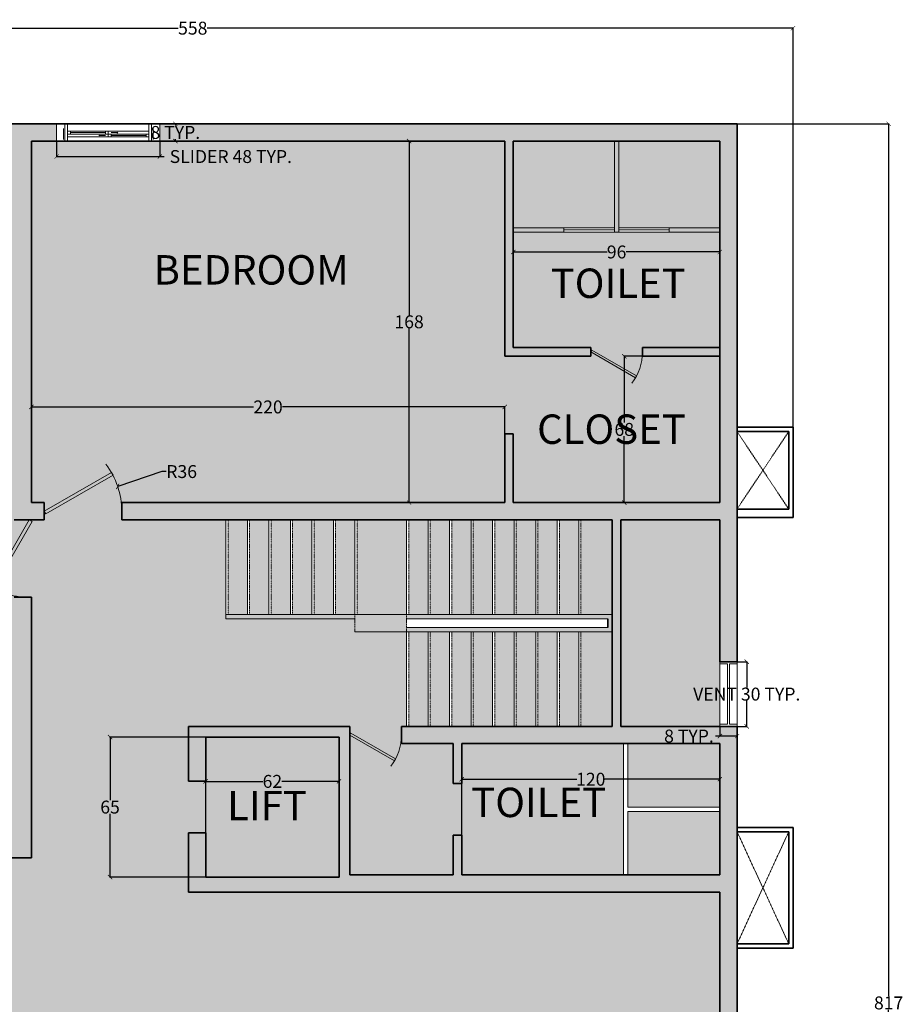
# Model space of a CAD drawing. Units: inches. Extents: x 1704 to 6393, y -157 to 1172.
# Tile 122 of 122: x 5982 to 6393, y 376 to 834. Entities that reach past the tile are written whole.
import ezdxf

# ---------------------------------------------------------------- set-up
doc = ezdxf.new("R2010")
doc.units = ezdxf.units.IN
doc.header["$MEASUREMENT"] = 0
doc.linetypes.add('DASHED', pattern=[0.75, 0.5, -0.25])
doc.linetypes.add('HIDDEN', pattern=[0.375, 0.25, -0.125])
for name, color, linetype, lineweight in [('A-ANNO-DIMS', 7, 'Continuous', 13), ('A-AREA-IDEN', 7, 'Continuous', 18), ('A-FLOR-OPEN-HIDN', 8, 'HIDDEN', 13), ('A-FLOR-STRS-HIDN', 8, 'DASHED', 13), ('A-GLAZ-PATT', 152, 'Continuous', 13), ('A-WALL-PATT', 7, 'Continuous', 13), ('DOORS', 160, 'Continuous', 18), ('GLASS PANEL FASADE', 4, 'Continuous', 18), ('STAIRS', 7, 'Continuous', 18), ('WALLS', 7, 'Continuous', 35), ('WINDOWS', 2, 'Continuous', 18)]:
    doc.layers.add(name, color=color, linetype=linetype, lineweight=lineweight)
doc.layers.add('A-FLOR-PATT', color=7, linetype='Continuous', lineweight=13, true_color=0xf2f2f2)
doc.styles.get("Standard").update_dxf_attribs({"font": 'arial.ttf'})
doc.dimstyles.get("Standard").update_dxf_attribs({"dimtxt": 6, "dimasz": 2, "dimexe": 0.18, "dimexo": 0.0625, "dimgap": 0.09, "dimtad": 0, "dimtih": 1, "dimtoh": 1, "dimdec": 1, "dimzin": 0, "dimdsep": 46, "dimlunit": 3, "dimtxsty": 'Standard', "dimblk": 'ARCHTICK', "dimcen": 0.09, "dimadec": 0, "dimazin": 0, "dimtfac": 1, "dimtdec": 1, "dimtofl": 0, "dimtmove": 0, "dimatfit": 3, "dimfxl": 1, "dimtolj": 1, "dimtzin": 0, "dimarcsym": 0})

# ---------------------------------------------------------------- blocks, each defined once
blk = doc.blocks.new('Door - Left Hung 36 in.')
blk.add_lwpolyline([(0.75, -1.3), (0, 0), (31.18, 18), (31.93, 16.7)], close=True)
blk.add_arc((0, 0), 36, 0, 37.3101)
blk = doc.blocks.new('WIN-SLIDER-48')
for p, q in [((3.83, 8), (0, 8)), ((3.18, 5.86), (3.18, 0.65)), ((5.13, 8), (42.87, 8)), ((44.17, 8), (48, 8)), ((44.82, 5.86), (44.82, 0.65)), ((24, 1.95), (5.13, 1.95)), ((6.43, 4.55), (22.7, 4.55)), ((6.43, 3.9), (22.7, 3.9)), ((6.43, 3.25), (22.7, 3.25)), ((22.7, 2.6), (19.9, 2.6)), ((24, 4.55), (42.87, 4.55)), ((25.3, 3.9), (28.1, 3.9)), ((25.3, 3.25), (41.56, 3.25)), ((25.3, 2.6), (41.56, 2.6)), ((25.3, 1.95), (41.56, 1.95)), ((3.83, 0), (0, 0)), ((5.13, 0), (42.87, 0)), ((44.17, 0), (48, 0))]:
    blk.add_line(p, q)
for points in [[(5.13, 0), (3.83, 0), (3.83, 8), (5.13, 8)], [(42.87, 0), (44.17, 0), (44.17, 8), (42.87, 8)], [(5.13, 3.25), (6.43, 3.25), (6.43, 4.55), (5.13, 4.55)], [(19.57, 2.6), (19.9, 2.8), (19.9, 2.41)], [(22.7, 3.25), (24, 3.25), (24, 4.55), (22.7, 4.55)], [(24, 1.95), (25.3, 1.95), (25.3, 3.25), (24, 3.25)], [(28.43, 3.9), (28.1, 4.1), (28.1, 3.71)], [(41.56, 1.95), (42.87, 1.95), (42.87, 3.25), (41.56, 3.25)]]:
    blk.add_lwpolyline(points, close=True)
blk = doc.blocks.new('WIN-VENT-30')
for p, q in [((0, 0), (0, 30)), ((0, 30), (8, 30)), ((0, 29), (3.5, 29)), ((3.5, 29), (3.5, 1)), ((4.5, 29), (8, 29)), ((4.5, 29), (4.5, 1)), ((8, 30), (8, 0)), ((3.5, 1), (0, 1)), ((8, 1), (4.5, 1)), ((8, 0), (0, 0))]:
    blk.add_line(p, q)
blk = doc.blocks.new('GLAZ-SHOWER-SCREEN-96')
for p, q in [((47, 2), (47, 42.3)), ((49, 2), (49, 42.3)), ((0, 2), (47, 2)), ((23.5, 2), (23.5, 0)), ((23.5, 1), (47, 1)), ((47, 2), (47, 0)), ((49, 2), (96, 2)), ((49, 2), (49, 0)), ((49, 1), (72.5, 1)), ((72.5, 2), (72.5, 0)), ((0, 0), (96, 0))]:
    blk.add_line(p, q)
blk = doc.blocks.new('_ArchTick')
at = {"color": 0, "linetype": 'ByBlock', "const_width": 0.15}
blk.add_lwpolyline([(-0.5, -0.5), (0.5, 0.5)], dxfattribs=at)
blk = doc.blocks.new('*D38')
at = {"layer": 'A-ANNO-DIMS', "color": 0, "lineweight": -2, "transparency": 16777216}
for p, q in [((5999.3, 777.42), (5999.3, 770.1)), ((6047.3, 777.42), (6047.3, 770.1)), ((5999.3, 770.28), (6047.3, 770.28)), ((6047.3, 770.28), (6049.3, 770.28))]:
    blk.add_line(p, q, dxfattribs=at)
at = {"layer": 'Defpoints', "color": 0, "lineweight": -3, "transparency": 16777216}
for p in [(5999.3, 777.48), (6047.3, 777.48), (6047.3, 770.28)]:
    blk.add_point(p, dxfattribs=at)
at = {"layer": 'A-ANNO-DIMS', "color": 0, "lineweight": -2, "transparency": 16777216, "xscale": 2, "yscale": 2, "zscale": 2, "rotation": 180}
blk.add_blockref('_ArchTick', (5999.3, 770.28), dxfattribs=at)
at = {"layer": 'A-ANNO-DIMS', "color": 0, "lineweight": -2, "transparency": 16777216, "xscale": 2, "yscale": 2, "zscale": 2}
blk.add_blockref('_ArchTick', (6047.3, 770.28), dxfattribs=at)
at = {"layer": 'A-ANNO-DIMS', "color": 0, "transparency": 16777216, "insert": (6080.28, 770.28), "char_height": 6, "attachment_point": 5}
blk.add_mtext('\\A1;SLIDER 48 TYP.', dxfattribs=at)
blk = doc.blocks.new('*D39')
at = {"layer": 'A-ANNO-DIMS', "color": 0, "lineweight": -2, "transparency": 16777216}
for p, q in [((6047.36, 785.48), (6054.68, 785.48)), ((6054.5, 785.48), (6054.5, 784.63)), ((6054.5, 777.48), (6054.5, 778.32)), ((6047.36, 777.48), (6054.68, 777.48))]:
    blk.add_line(p, q, dxfattribs=at)
at = {"layer": 'Defpoints', "color": 0, "lineweight": -3, "transparency": 16777216}
for p in [(6047.3, 785.48), (6054.5, 785.48), (6047.3, 777.48)]:
    blk.add_point(p, dxfattribs=at)
at = {"layer": 'A-ANNO-DIMS', "color": 0, "lineweight": -2, "transparency": 16777216, "xscale": 2, "yscale": 2, "zscale": 2}
for p, rotation in [((6054.5, 785.48), 90), ((6054.5, 777.48), 270)]:
    blk.add_blockref('_ArchTick', p, dxfattribs=dict(at, rotation=rotation))
at = {"layer": 'A-ANNO-DIMS', "color": 0, "transparency": 16777216, "insert": (6054.5, 781.48), "char_height": 6, "attachment_point": 5}
blk.add_mtext('\\A1;8 TYP.', dxfattribs=at)
blk = doc.blocks.new('*D44')
at = {"layer": 'A-ANNO-DIMS', "color": 0, "lineweight": -2, "transparency": 16777216}
for p, q in [((6315.65, 535.48), (6320.27, 535.48)), ((6320.09, 535.48), (6320.09, 523.63)), ((6320.09, 505.48), (6320.09, 517.32)), ((6315.65, 505.48), (6320.27, 505.48))]:
    blk.add_line(p, q, dxfattribs=at)
at = {"layer": 'Defpoints', "color": 0, "lineweight": -3, "transparency": 16777216}
for p in [(6315.59, 535.48), (6315.59, 505.48), (6320.09, 505.48)]:
    blk.add_point(p, dxfattribs=at)
at = {"layer": 'A-ANNO-DIMS', "color": 0, "lineweight": -2, "transparency": 16777216, "xscale": 2, "yscale": 2, "zscale": 2}
for p, rotation in [((6320.09, 535.48), 90), ((6320.09, 505.48), 270)]:
    blk.add_blockref('_ArchTick', p, dxfattribs=dict(at, rotation=rotation))
at = {"layer": 'A-ANNO-DIMS', "color": 0, "transparency": 16777216, "insert": (6320.09, 520.48), "char_height": 6, "attachment_point": 5}
blk.add_mtext('\\A1;VENT 30 TYP.', dxfattribs=at)
blk = doc.blocks.new('*D45')
at = {"layer": 'A-ANNO-DIMS', "color": 0, "lineweight": -2, "transparency": 16777216}
for p, q in [((6307.59, 505.42), (6307.59, 500.8)), ((6315.59, 505.42), (6315.59, 500.8)), ((6307.59, 500.98), (6305.59, 500.98)), ((6315.59, 500.98), (6307.59, 500.98))]:
    blk.add_line(p, q, dxfattribs=at)
at = {"layer": 'Defpoints', "color": 0, "lineweight": -3, "transparency": 16777216}
for p in [(6307.59, 505.48), (6315.59, 505.48), (6307.59, 500.98)]:
    blk.add_point(p, dxfattribs=at)
at = {"layer": 'A-ANNO-DIMS', "color": 0, "lineweight": -2, "transparency": 16777216, "xscale": 2, "yscale": 2, "zscale": 2, "rotation": 180}
blk.add_blockref('_ArchTick', (6307.59, 500.98), dxfattribs=at)
at = {"layer": 'A-ANNO-DIMS', "color": 0, "lineweight": -2, "transparency": 16777216, "xscale": 2, "yscale": 2, "zscale": 2}
blk.add_blockref('_ArchTick', (6315.59, 500.98), dxfattribs=at)
at = {"layer": 'A-ANNO-DIMS', "color": 0, "transparency": 16777216, "insert": (6293.22, 500.98), "char_height": 6, "attachment_point": 5}
blk.add_mtext('\\A1;8 TYP.', dxfattribs=at)
blk = doc.blocks.new('*D119')
at = {"layer": 'A-ANNO-DIMS', "color": 0, "lineweight": -2, "transparency": 16777216}
for p, q in [((5783.59, 785.54), (5783.59, 830.11)), ((5783.59, 829.93), (6055.87, 829.93)), ((6341.59, 829.93), (6069.31, 829.93)), ((6341.59, 644.54), (6341.59, 830.11))]:
    blk.add_line(p, q, dxfattribs=at)
at = {"layer": 'Defpoints', "color": 0, "lineweight": -3, "transparency": 16777216}
for p in [(6341.59, 829.93), (5783.59, 785.48), (6341.59, 644.48)]:
    blk.add_point(p, dxfattribs=at)
at = {"layer": 'A-ANNO-DIMS', "color": 0, "lineweight": -2, "transparency": 16777216, "xscale": 2, "yscale": 2, "zscale": 2, "rotation": 180}
blk.add_blockref('_ArchTick', (5783.59, 829.93), dxfattribs=at)
at = {"layer": 'A-ANNO-DIMS', "color": 0, "lineweight": -2, "transparency": 16777216, "xscale": 2, "yscale": 2, "zscale": 2}
blk.add_blockref('_ArchTick', (6341.59, 829.93), dxfattribs=at)
at = {"layer": 'A-ANNO-DIMS', "color": 0, "transparency": 16777216, "insert": (6062.59, 829.93), "char_height": 6, "attachment_point": 5}
blk.add_mtext('\\A1;558', dxfattribs=at)
blk = doc.blocks.new('*D120')
at = {"layer": 'A-ANNO-DIMS', "color": 0, "lineweight": -2, "transparency": 16777216}
for p, q in [((6315.65, 785.48), (6386.22, 785.48)), ((6386.04, 785.48), (6386.04, 380.13)), ((6386.04, -31.52), (6386.04, 373.82)), ((6315.65, -31.52), (6386.22, -31.52))]:
    blk.add_line(p, q, dxfattribs=at)
at = {"layer": 'Defpoints', "color": 0, "lineweight": -3, "transparency": 16777216}
for p in [(6315.59, 785.48), (6315.59, -31.52), (6386.04, -31.52)]:
    blk.add_point(p, dxfattribs=at)
at = {"layer": 'A-ANNO-DIMS', "color": 0, "lineweight": -2, "transparency": 16777216, "xscale": 2, "yscale": 2, "zscale": 2}
for p, rotation in [((6386.04, 785.48), 90), ((6386.04, -31.52), 270)]:
    blk.add_blockref('_ArchTick', p, dxfattribs=dict(at, rotation=rotation))
at = {"layer": 'A-ANNO-DIMS', "color": 0, "transparency": 16777216, "insert": (6386.04, 376.98), "char_height": 6, "attachment_point": 5}
blk.add_mtext('\\A1;817', dxfattribs=at)
blk = doc.blocks.new('*D127')
at = {"layer": 'A-ANNO-DIMS', "color": 0, "lineweight": -2, "transparency": 16777216}
for p, q in [((5987.59, 609.54), (5987.59, 654.11)), ((5987.59, 653.93), (6090.83, 653.93)), ((6207.59, 653.93), (6104.35, 653.93)), ((6207.59, 609.54), (6207.59, 654.11))]:
    blk.add_line(p, q, dxfattribs=at)
at = {"layer": 'Defpoints', "color": 0, "lineweight": -3, "transparency": 16777216}
for p in [(6207.59, 653.93), (5987.59, 609.48), (6207.59, 609.48)]:
    blk.add_point(p, dxfattribs=at)
at = {"layer": 'A-ANNO-DIMS', "color": 0, "lineweight": -2, "transparency": 16777216, "xscale": 2, "yscale": 2, "zscale": 2, "rotation": 180}
blk.add_blockref('_ArchTick', (5987.59, 653.93), dxfattribs=at)
at = {"layer": 'A-ANNO-DIMS', "color": 0, "lineweight": -2, "transparency": 16777216, "xscale": 2, "yscale": 2, "zscale": 2}
blk.add_blockref('_ArchTick', (6207.59, 653.93), dxfattribs=at)
at = {"layer": 'A-ANNO-DIMS', "color": 0, "transparency": 16777216, "insert": (6097.59, 653.93), "char_height": 6, "attachment_point": 5}
blk.add_mtext('\\A1;220', dxfattribs=at)
blk = doc.blocks.new('*D128')
at = {"layer": 'A-ANNO-DIMS', "color": 0, "lineweight": -2, "transparency": 16777216}
for p, q in [((6207.53, 777.48), (6162.96, 777.48)), ((6163.14, 777.48), (6163.14, 696.63)), ((6163.14, 609.48), (6163.14, 690.32)), ((6207.53, 609.48), (6162.96, 609.48))]:
    blk.add_line(p, q, dxfattribs=at)
at = {"layer": 'Defpoints', "color": 0, "lineweight": -3, "transparency": 16777216}
for p in [(6163.14, 777.48), (6207.59, 777.48), (6207.59, 609.48)]:
    blk.add_point(p, dxfattribs=at)
at = {"layer": 'A-ANNO-DIMS', "color": 0, "lineweight": -2, "transparency": 16777216, "xscale": 2, "yscale": 2, "zscale": 2}
for p, rotation in [((6163.14, 777.48), 90), ((6163.14, 609.48), 270)]:
    blk.add_blockref('_ArchTick', p, dxfattribs=dict(at, rotation=rotation))
at = {"layer": 'A-ANNO-DIMS', "color": 0, "transparency": 16777216, "insert": (6163.14, 693.48), "char_height": 6, "attachment_point": 5}
blk.add_mtext('\\A1;168', dxfattribs=at)
blk = doc.blocks.new('*D131')
at = {"layer": 'A-ANNO-DIMS', "color": 0, "lineweight": -2, "transparency": 16777216}
for p, q in [((6211.59, 681.54), (6211.59, 726.11)), ((6211.59, 725.93), (6255.2, 725.93)), ((6307.59, 725.93), (6263.98, 725.93)), ((6307.59, 681.54), (6307.59, 726.11))]:
    blk.add_line(p, q, dxfattribs=at)
at = {"layer": 'Defpoints', "color": 0, "lineweight": -3, "transparency": 16777216}
for p in [(6307.59, 725.93), (6211.59, 681.48), (6307.59, 681.48)]:
    blk.add_point(p, dxfattribs=at)
at = {"layer": 'A-ANNO-DIMS', "color": 0, "lineweight": -2, "transparency": 16777216, "xscale": 2, "yscale": 2, "zscale": 2, "rotation": 180}
blk.add_blockref('_ArchTick', (6211.59, 725.93), dxfattribs=at)
at = {"layer": 'A-ANNO-DIMS', "color": 0, "lineweight": -2, "transparency": 16777216, "xscale": 2, "yscale": 2, "zscale": 2}
blk.add_blockref('_ArchTick', (6307.59, 725.93), dxfattribs=at)
at = {"layer": 'A-ANNO-DIMS', "color": 0, "transparency": 16777216, "insert": (6259.59, 725.93), "char_height": 6, "attachment_point": 5}
blk.add_mtext('\\A1;96', dxfattribs=at)
blk = doc.blocks.new('*D132')
at = {"layer": 'A-ANNO-DIMS', "color": 0, "lineweight": -2, "transparency": 16777216}
for p, q in [((6307.53, 677.48), (6262.96, 677.48)), ((6263.14, 677.48), (6263.14, 646.63)), ((6263.14, 609.48), (6263.14, 640.32)), ((6307.53, 609.48), (6262.96, 609.48))]:
    blk.add_line(p, q, dxfattribs=at)
at = {"layer": 'Defpoints', "color": 0, "lineweight": -3, "transparency": 16777216}
for p in [(6263.14, 677.48), (6307.59, 677.48), (6307.59, 609.48)]:
    blk.add_point(p, dxfattribs=at)
at = {"layer": 'A-ANNO-DIMS', "color": 0, "lineweight": -2, "transparency": 16777216, "xscale": 2, "yscale": 2, "zscale": 2}
for p, rotation in [((6263.14, 677.48), 90), ((6263.14, 609.48), 270)]:
    blk.add_blockref('_ArchTick', p, dxfattribs=dict(at, rotation=rotation))
at = {"layer": 'A-ANNO-DIMS', "color": 0, "transparency": 16777216, "insert": (6263.14, 643.48), "char_height": 6, "attachment_point": 5}
blk.add_mtext('\\A1;68', dxfattribs=at)
blk = doc.blocks.new('*D133')
at = {"layer": 'A-ANNO-DIMS', "color": 0, "lineweight": -2, "transparency": 16777216}
for p, q in [((6187.59, 436.54), (6187.59, 481.11)), ((6187.59, 480.93), (6241.16, 480.93)), ((6307.59, 480.93), (6254.02, 480.93)), ((6307.59, 436.54), (6307.59, 481.11))]:
    blk.add_line(p, q, dxfattribs=at)
at = {"layer": 'Defpoints', "color": 0, "lineweight": -3, "transparency": 16777216}
for p in [(6307.59, 480.93), (6187.59, 436.48), (6307.59, 436.48)]:
    blk.add_point(p, dxfattribs=at)
at = {"layer": 'A-ANNO-DIMS', "color": 0, "lineweight": -2, "transparency": 16777216, "xscale": 2, "yscale": 2, "zscale": 2, "rotation": 180}
blk.add_blockref('_ArchTick', (6187.59, 480.93), dxfattribs=at)
at = {"layer": 'A-ANNO-DIMS', "color": 0, "lineweight": -2, "transparency": 16777216, "xscale": 2, "yscale": 2, "zscale": 2}
blk.add_blockref('_ArchTick', (6307.59, 480.93), dxfattribs=at)
at = {"layer": 'A-ANNO-DIMS', "color": 0, "transparency": 16777216, "insert": (6247.59, 480.93), "char_height": 6, "attachment_point": 5}
blk.add_mtext('\\A1;120', dxfattribs=at)
blk = doc.blocks.new('*D134')
at = {"layer": 'A-ANNO-DIMS', "color": 0, "lineweight": -2, "transparency": 16777216}
for p, q in [((6068.59, 435.54), (6068.59, 480.11)), ((6068.59, 479.93), (6095.22, 479.93)), ((6130.59, 479.93), (6103.96, 479.93)), ((6130.59, 435.54), (6130.59, 480.11))]:
    blk.add_line(p, q, dxfattribs=at)
at = {"layer": 'Defpoints', "color": 0, "lineweight": -3, "transparency": 16777216}
for p in [(6130.59, 479.93), (6068.59, 435.48), (6130.59, 435.48)]:
    blk.add_point(p, dxfattribs=at)
at = {"layer": 'A-ANNO-DIMS', "color": 0, "lineweight": -2, "transparency": 16777216, "xscale": 2, "yscale": 2, "zscale": 2, "rotation": 180}
blk.add_blockref('_ArchTick', (6068.59, 479.93), dxfattribs=at)
at = {"layer": 'A-ANNO-DIMS', "color": 0, "lineweight": -2, "transparency": 16777216, "xscale": 2, "yscale": 2, "zscale": 2}
blk.add_blockref('_ArchTick', (6130.59, 479.93), dxfattribs=at)
at = {"layer": 'A-ANNO-DIMS', "color": 0, "transparency": 16777216, "insert": (6099.59, 479.93), "char_height": 6, "attachment_point": 5}
blk.add_mtext('\\A1;62', dxfattribs=at)
blk = doc.blocks.new('*D135')
at = {"layer": 'A-ANNO-DIMS', "color": 0, "lineweight": -2, "transparency": 16777216}
for p, q in [((6068.53, 500.48), (6023.96, 500.48)), ((6024.14, 500.48), (6024.14, 471.13)), ((6024.14, 435.48), (6024.14, 464.82)), ((6068.53, 435.48), (6023.96, 435.48))]:
    blk.add_line(p, q, dxfattribs=at)
at = {"layer": 'Defpoints', "color": 0, "lineweight": -3, "transparency": 16777216}
for p in [(6024.14, 500.48), (6068.59, 500.48), (6068.59, 435.48)]:
    blk.add_point(p, dxfattribs=at)
at = {"layer": 'A-ANNO-DIMS', "color": 0, "lineweight": -2, "transparency": 16777216, "xscale": 2, "yscale": 2, "zscale": 2}
for p, rotation in [((6024.14, 500.48), 90), ((6024.14, 435.48), 270)]:
    blk.add_blockref('_ArchTick', p, dxfattribs=dict(at, rotation=rotation))
at = {"layer": 'A-ANNO-DIMS', "color": 0, "transparency": 16777216, "insert": (6024.14, 467.98), "char_height": 6, "attachment_point": 5}
blk.add_mtext('\\A1;65', dxfattribs=at)
blk = doc.blocks.new('*D139')
at = {"layer": 'A-ANNO-DIMS', "color": 0, "lineweight": -2, "transparency": 16777216}
for p, q in [((6048.16, 623.9), (6027.7, 616.99)), ((6050.16, 623.9), (6048.16, 623.9)), ((5993.5, 605.48), (5993.68, 605.48)), ((5993.59, 605.39), (5993.59, 605.57))]:
    blk.add_line(p, q, dxfattribs=at)
at = {"layer": 'Defpoints', "color": 0, "lineweight": -3, "transparency": 16777216}
for p in [(6027.7, 616.99), (5993.59, 605.48)]:
    blk.add_point(p, dxfattribs=at)
at = {"layer": 'A-ANNO-DIMS', "color": 0, "lineweight": -2, "transparency": 16777216, "xscale": 2, "yscale": 2, "zscale": 2, "rotation": 198.6542347381252}
blk.add_blockref('_ArchTick', (6027.7, 616.99), dxfattribs=at)
at = {"layer": 'A-ANNO-DIMS', "color": 0, "transparency": 16777216, "insert": (6057.42, 623.9), "char_height": 6, "attachment_point": 5}
blk.add_mtext('\\A1;R36', dxfattribs=at)

msp = doc.modelspace()

# ---------------------------------------------------------------- hatches: boundary and pattern name
at = {"layer": 'A-FLOR-PATT', "transparency": 33554559}
h = msp.add_hatch(color=256, dxfattribs=at)
h.dxf.hatch_style = 1
h.paths.add_polyline_path([(5979.59, 777.478), (5791.59, 777.478), (5791.59, 741.478), (5979.59, 741.478)], flags=17)
h.paths.add_polyline_path([(5979.59, 733.478), (5791.59, 733.478), (5791.59, 565.478), (5907.59, 565.478), (5907.59, 561.478), (5883.59, 561.478), (5883.59, 555.478), (5875.59, 555.478), (5875.59, 561.478), (5791.59, 561.478), (5791.59, 452.478), (5875.59, 452.478), (5875.59, 525.478), (5883.59, 525.478), (5883.59, 452.478), (5979.59, 452.478), (5979.59, 561.478), (5943.59, 561.478), (5943.59, 565.478), (5979.59, 565.478), (5987.59, 565.478), (5987.59, 444.478), (5791.59, 444.478), (5791.603, 92.478), (6059.59, 92.478), (6059.59, 292.478), (6101.682, 292.478), (6101.682, 284.478), (6067.59, 284.478), (6067.59, 164.478), (6079.59, 164.478), (6079.59, 156.478), (6067.59, 156.478), (6067.59, -11.522), (6307.59, -11.522), (6307.59, 108.478), (6307.59, 117.524), (6307.59, 156.478), (6115.59, 156.478), (6115.59, 164.478), (6307.59, 164.478), (6307.59, 236.478), (6307.59, 262.478), (6307.59, 284.478), (6137.682, 284.478), (6137.682, 292.478), (6307.59, 292.478), (6307.59, 428.478), (6068.59, 428.478), (6060.59, 428.478), (6060.59, 455.978), (6068.59, 455.978), (6068.59, 435.478), (6130.59, 435.478), (6130.59, 500.478), (6068.59, 500.478), (6068.59, 479.978), (6060.59, 479.978), (6060.59, 505.478), (6135.59, 505.478), (6135.59, 497.478), (6135.59, 436.478), (6183.59, 436.478), (6183.59, 454.978), (6187.59, 454.978), (6187.59, 436.478), (6262.788, 436.478), (6262.788, 497.478), (6187.59, 497.478), (6187.59, 478.978), (6183.59, 478.978), (6183.59, 497.478), (6159.59, 497.478), (6159.59, 505.478), (6161.98, 505.478), (6161.98, 549.478), (6137.98, 549.478), (6137.98, 555.478), (6077.98, 555.478), (6077.98, 557.478), (6077.98, 601.478), (6029.59, 601.478), (6029.59, 609.478), (6035.59, 609.478), (6207.59, 609.478), (6207.59, 641.478), (6211.59, 641.478), (6211.59, 609.478), (6223.59, 609.478), (6307.59, 609.478), (6307.59, 677.478), (6271.59, 677.478), (6271.59, 681.478), (6307.59, 681.478), (6307.59, 735.174), (6211.59, 735.174), (6211.59, 681.478), (6247.59, 681.478), (6247.59, 677.478), (6211.59, 677.478), (6207.59, 677.478), (6207.59, 777.478), (5987.59, 777.478), (5987.59, 609.478), (5993.59, 609.478), (5993.59, 601.478), (5979.59, 601.478)])
h.paths.add_polyline_path([(6307.59, 601.478), (6261.59, 601.478), (6261.59, 505.478), (6307.59, 505.478), (6307.59, 535.478)], flags=17)
h.paths.add_polyline_path([(6161.98, 601.478), (6138.98, 601.478), (6138.98, 557.478), (6161.98, 557.478)], flags=17)
h.paths.add_polyline_path([(6257.59, 601.478), (6242.98, 601.478), (6242.98, 557.478), (6257.59, 557.478)], flags=17)
h.paths.add_polyline_path([(6117.98, 601.478), (6108.98, 601.478), (6108.98, 557.478), (6117.98, 557.478)], flags=17)
h.paths.add_polyline_path([(6107.98, 601.478), (6098.98, 601.478), (6098.98, 557.478), (6107.98, 557.478)], flags=17)
h.paths.add_polyline_path([(6097.98, 601.478), (6088.98, 601.478), (6088.98, 557.478), (6097.98, 557.478)], flags=17)
h.paths.add_polyline_path([(6087.98, 601.478), (6078.98, 601.478), (6078.98, 557.478), (6087.98, 557.478)], flags=17)
h.paths.add_polyline_path([(6127.98, 601.478), (6118.98, 601.478), (6118.98, 557.478), (6127.98, 557.478)], flags=17)
h.paths.add_polyline_path([(6137.98, 601.478), (6128.98, 601.478), (6128.98, 557.478), (6137.98, 557.478)], flags=17)
h.paths.add_polyline_path([(6171.98, 601.478), (6162.98, 601.478), (6162.98, 557.478), (6171.98, 557.478)], flags=17)
h.paths.add_polyline_path([(6181.98, 601.478), (6172.98, 601.478), (6172.98, 557.478), (6181.98, 557.478)], flags=17)
h.paths.add_polyline_path([(6191.98, 601.478), (6182.98, 601.478), (6182.98, 557.478), (6191.98, 557.478)], flags=17)
h.paths.add_polyline_path([(6201.98, 601.478), (6192.98, 601.478), (6192.98, 557.478), (6201.98, 557.478)], flags=17)
h.paths.add_polyline_path([(6211.98, 601.478), (6202.98, 601.478), (6202.98, 557.478), (6211.98, 557.478)], flags=17)
h.paths.add_polyline_path([(6221.98, 601.478), (6212.98, 601.478), (6212.98, 557.478), (6221.98, 557.478)], flags=17)
h.paths.add_polyline_path([(6231.98, 601.478), (6222.98, 601.478), (6222.98, 557.478), (6231.98, 557.478)], flags=17)
h.paths.add_polyline_path([(6241.98, 601.478), (6232.98, 601.478), (6232.98, 557.478), (6241.98, 557.478)], flags=17)
h.paths.add_polyline_path([(6171.98, 549.478), (6162.98, 549.478), (6162.98, 505.478), (6171.98, 505.478)], flags=17)
h.paths.add_polyline_path([(6181.98, 549.478), (6172.98, 549.478), (6172.98, 505.478), (6181.98, 505.478)], flags=17)
h.paths.add_polyline_path([(6191.98, 549.478), (6182.98, 549.478), (6182.98, 505.478), (6191.98, 505.478)], flags=17)
h.paths.add_polyline_path([(6201.98, 549.478), (6192.98, 549.478), (6192.98, 505.478), (6201.98, 505.478)], flags=17)
h.paths.add_polyline_path([(6211.98, 549.478), (6202.98, 549.478), (6202.98, 505.478), (6211.98, 505.478)], flags=17)
h.paths.add_polyline_path([(6221.98, 549.478), (6212.98, 549.478), (6212.98, 505.478), (6221.98, 505.478)], flags=17)
h.paths.add_polyline_path([(6231.98, 549.478), (6222.98, 549.478), (6222.98, 505.478), (6231.98, 505.478)], flags=17)
h.paths.add_polyline_path([(6241.98, 549.478), (6232.98, 549.478), (6232.98, 505.478), (6241.98, 505.478)], flags=17)
h.paths.add_polyline_path([(6257.59, 549.478), (6242.98, 549.478), (6242.98, 505.478), (6257.59, 505.478)], flags=17)
h = msp.add_hatch(color=256, dxfattribs=at)
h.dxf.hatch_style = 1
h.paths.add_polyline_path([(6258.59, 777.478), (6211.59, 777.478), (6211.59, 737.174), (6258.59, 737.174)])
h.paths.add_polyline_path([(6307.59, 777.478), (6260.59, 777.478), (6260.59, 737.174), (6307.59, 737.174)])
h = msp.add_hatch(color=256, dxfattribs=at)
h.dxf.hatch_style = 1
h.paths.add_polyline_path([(6307.59, 497.478), (6264.788, 497.478), (6264.788, 467.978), (6307.59, 467.978)])
h.paths.add_polyline_path([(6307.59, 465.978), (6264.788, 465.978), (6264.788, 436.478), (6307.59, 436.478)])
at = {"layer": 'A-GLAZ-PATT', "transparency": 33554559}
h = msp.add_hatch(color=256, dxfattribs=at)
h.dxf.hatch_style = 1
h.paths.add_polyline_path([(6235.09, 737.174), (6211.59, 737.174), (6211.59, 735.174), (6235.09, 735.174)])
h.paths.add_polyline_path([(6260.59, 777.478), (6258.59, 777.478), (6258.59, 737.174), (6258.59, 735.174), (6260.59, 735.174), (6260.59, 737.174)])
h = msp.add_hatch(color=256, dxfattribs=at)
h.dxf.hatch_style = 1
h.paths.add_polyline_path([(6307.59, 737.174), (6284.09, 737.174), (6284.09, 735.174), (6307.59, 735.174)])
at = {"layer": 'A-WALL-PATT', "transparency": 33554559}
h = msp.add_hatch(color=256, dxfattribs=at)
h.dxf.hatch_style = 1
h.paths.add_polyline_path([(5791.59, 733.478), (5837.59, 733.478), (5837.59, 741.478), (5791.59, 741.478), (5791.59, 777.478), (5803.735, 777.478), (5803.735, 785.478), (5783.59, 785.478), (5783.59, 637.478), (5791.59, 637.478)])
h.paths.add_polyline_path([(5987.59, 777.478), (5999.299, 777.478), (5999.299, 785.478), (5983.59, 785.478), (5967.445, 785.478), (5967.445, 777.478), (5979.59, 777.478), (5979.59, 741.478), (5933.59, 741.478), (5933.59, 733.478), (5979.59, 733.478), (5979.59, 601.478), (5993.59, 601.478), (5993.59, 609.478), (5987.59, 609.478)])
h = msp.add_hatch(color=256, dxfattribs=at)
h.dxf.hatch_style = 1
h.paths.add_polyline_path([(6315.59, 785.478), (6047.299, 785.478), (6047.299, 777.478), (6207.59, 777.478), (6207.59, 677.478), (6211.59, 677.478), (6247.59, 677.478), (6247.59, 681.478), (6211.59, 681.478), (6211.59, 777.478), (6307.59, 777.478), (6307.59, 744.478), (6307.59, 677.478), (6307.59, 609.478), (6211.59, 609.478), (6211.59, 641.478), (6207.59, 641.478), (6207.59, 609.478), (6035.59, 609.478), (6029.59, 609.478), (6029.59, 601.478), (6257.59, 601.478), (6257.59, 505.478), (6159.59, 505.478), (6159.59, 497.478), (6183.59, 497.478), (6183.59, 478.978), (6187.59, 478.978), (6187.59, 497.478), (6307.59, 497.478), (6307.59, 436.478), (6187.59, 436.478), (6187.59, 454.978), (6183.59, 454.978), (6183.59, 436.478), (6135.59, 436.478), (6135.59, 497.478), (6135.59, 505.478), (6060.59, 505.478), (6060.59, 479.978), (6068.59, 479.978), (6068.59, 500.478), (6130.59, 500.478), (6130.59, 435.478), (6068.59, 435.478), (6068.59, 455.978), (6060.59, 455.978), (6060.59, 428.478), (6187.59, 428.478), (6307.59, 428.478), (6307.59, 385.478), (6307.59, 363.289), (6315.59, 363.289), (6315.59, 402.478), (6315.59, 404.478), (6315.59, 456.478), (6315.59, 458.478), (6315.59, 497.478), (6315.59, 505.478), (6307.59, 505.478), (6261.59, 505.478), (6261.59, 601.478), (6307.59, 601.478), (6307.59, 535.478), (6315.59, 535.478), (6315.59, 602.478), (6315.59, 606.478), (6315.59, 642.478), (6315.59, 644.478)])
h.paths.add_polyline_path([(5791.59, 561.478), (5875.59, 561.478), (5875.59, 555.478), (5883.59, 555.478), (5883.59, 561.478), (5907.59, 561.478), (5907.59, 565.478), (5791.59, 565.478), (5783.59, 565.478), (5783.59, 444.478), (5987.59, 444.478), (5987.59, 565.478), (5979.59, 565.478), (5943.59, 565.478), (5943.59, 561.478), (5979.59, 561.478), (5979.59, 452.478), (5883.59, 452.478), (5883.59, 525.478), (5875.59, 525.478), (5875.59, 452.478), (5791.59, 452.478)])
h = msp.add_hatch(color=256, dxfattribs=at)
h.dxf.hatch_style = 1
h.paths.add_polyline_path([(6307.59, 681.478), (6271.59, 681.478), (6271.59, 677.478), (6307.59, 677.478)])
h = msp.add_hatch(color=256, dxfattribs=at)
h.dxf.hatch_style = 1
h.paths.add_polyline_path([(6161.98, 557.478), (6137.98, 557.478), (6137.98, 549.478), (6161.98, 549.478)])
h.paths.add_polyline_path([(6137.98, 557.478), (6077.98, 557.478), (6077.98, 555.478), (6137.98, 555.478)])
h.paths.add_polyline_path([(6257.59, 557.478), (6161.98, 557.478), (6161.98, 555.478), (6255.59, 555.478), (6255.59, 551.478), (6161.98, 551.478), (6161.98, 549.478), (6257.59, 549.478)])

# ---------------------------------------------------------------- linework, layer by layer
at = {"layer": 'A-FLOR-OPEN-HIDN'}
for p, q in [((6315.59, 606.478), (6339.59, 642.478)), ((6315.59, 642.478), (6339.59, 606.478)), ((6315.59, 404.478), (6339.59, 456.478)), ((6315.59, 456.478), (6339.59, 404.478))]:
    msp.add_line(p, q, dxfattribs=at)
at = {"layer": 'A-FLOR-STRS-HIDN'}
for p, q in [((6078.98, 557.478), (6078.98, 601.478)), ((6088.98, 557.478), (6088.98, 601.478)), ((6098.98, 557.478), (6098.98, 601.478)), ((6108.98, 557.478), (6108.98, 601.478)), ((6118.98, 557.478), (6118.98, 601.478)), ((6128.98, 557.478), (6128.98, 601.478)), ((6138.98, 557.478), (6138.98, 601.478)), ((6162.98, 557.478), (6162.98, 601.478)), ((6172.98, 557.478), (6172.98, 601.478)), ((6182.98, 557.478), (6182.98, 601.478)), ((6192.98, 557.478), (6192.98, 601.478)), ((6202.98, 557.478), (6202.98, 601.478)), ((6212.98, 557.478), (6212.98, 601.478)), ((6222.98, 557.478), (6222.98, 601.478)), ((6232.98, 557.478), (6232.98, 601.478)), ((6242.98, 557.478), (6242.98, 601.478)), ((6137.98, 557.478), (6137.98, 549.478)), ((6161.98, 549.478), (6161.98, 557.478)), ((6162.98, 549.478), (6162.98, 505.478)), ((6172.98, 549.478), (6172.98, 505.478)), ((6182.98, 549.478), (6182.98, 505.478)), ((6192.98, 549.478), (6192.98, 505.478)), ((6202.98, 549.478), (6202.98, 505.478)), ((6212.98, 549.478), (6212.98, 505.478)), ((6222.98, 549.478), (6222.98, 505.478)), ((6232.98, 549.478), (6232.98, 505.478)), ((6242.98, 549.478), (6242.98, 505.478))]:
    msp.add_line(p, q, dxfattribs=at)
at = {"layer": 'GLASS PANEL FASADE'}
for p, q in [((6262.788, 436.478), (6262.788, 497.478)), ((6264.788, 467.978), (6264.788, 497.478)), ((6264.788, 467.978), (6307.59, 467.978)), ((6264.788, 436.478), (6264.788, 465.978)), ((6264.788, 465.978), (6307.59, 465.978))]:
    msp.add_line(p, q, dxfattribs=at)
at = {"layer": 'STAIRS'}
for p, q in [((6077.98, 557.478), (6077.98, 601.478)), ((6087.98, 557.478), (6087.98, 601.478)), ((6097.98, 557.478), (6097.98, 601.478)), ((6107.98, 557.478), (6107.98, 601.478)), ((6117.98, 557.478), (6117.98, 601.478)), ((6127.98, 557.478), (6127.98, 601.478)), ((6137.98, 557.478), (6137.98, 601.478)), ((6161.98, 557.478), (6161.98, 601.478)), ((6171.98, 557.478), (6171.98, 601.478)), ((6181.98, 557.478), (6181.98, 601.478)), ((6191.98, 557.478), (6191.98, 601.478)), ((6201.98, 557.478), (6201.98, 601.478)), ((6211.98, 557.478), (6211.98, 601.478)), ((6221.98, 557.478), (6221.98, 601.478)), ((6231.98, 557.478), (6231.98, 601.478)), ((6241.98, 557.478), (6241.98, 601.478)), ((6257.59, 557.478), (6077.98, 557.478)), ((6077.98, 555.478), (6077.98, 557.478)), ((6137.98, 555.478), (6077.98, 555.478)), ((6255.59, 555.478), (6161.98, 555.478)), ((6257.59, 549.478), (6137.98, 549.478)), ((6255.59, 551.478), (6161.98, 551.478)), ((6161.98, 549.478), (6161.98, 505.478)), ((6171.98, 549.478), (6171.98, 505.478)), ((6181.98, 549.478), (6181.98, 505.478)), ((6191.98, 549.478), (6191.98, 505.478)), ((6201.98, 549.478), (6201.98, 505.478)), ((6211.98, 549.478), (6211.98, 505.478)), ((6221.98, 549.478), (6221.98, 505.478)), ((6231.98, 549.478), (6231.98, 505.478)), ((6241.98, 549.478), (6241.98, 505.478))]:
    msp.add_line(p, q, dxfattribs=at)
at = {"layer": 'WALLS'}
for p, q in [((6315.59, 785.478), (5783.59, 785.478)), ((6315.59, 785.478), (5983.59, 785.478)), ((6315.59, 785.478), (6291.59, 785.478)), ((6315.59, 644.478), (6315.59, 785.478)), ((6315.59, 744.478), (6315.59, 785.478)), ((5987.59, 609.478), (5987.59, 777.478)), ((6207.59, 777.478), (5987.59, 777.478)), ((6207.59, 777.478), (6043.59, 777.478)), ((6207.59, 677.478), (6207.59, 777.478)), ((6211.59, 681.478), (6211.59, 777.478)), ((6211.59, 681.478), (6211.59, 777.478)), ((6307.59, 777.478), (6211.59, 777.478)), ((6307.59, 777.478), (6291.59, 777.478)), ((6307.59, 677.478), (6307.59, 777.478)), ((6307.59, 744.478), (6307.59, 777.478)), ((6307.59, 609.478), (6307.59, 708.478)), ((6211.59, 677.478), (6207.59, 677.478)), ((6247.59, 681.478), (6211.59, 681.478)), ((6247.59, 677.478), (6211.59, 677.478)), ((6247.59, 677.478), (6247.59, 681.478)), ((6307.59, 681.478), (6271.59, 681.478)), ((6271.59, 677.478), (6271.59, 681.478)), ((6307.59, 677.478), (6271.59, 677.478)), ((6207.59, 609.478), (6207.59, 641.478)), ((6211.59, 641.478), (6207.59, 641.478)), ((6211.59, 609.478), (6211.59, 641.478)), ((6315.59, 644.478), (6341.59, 644.478)), ((6315.59, 644.478), (6315.59, 642.478)), ((6315.59, 606.478), (6315.59, 642.478)), ((6315.59, 642.478), (6339.59, 642.478)), ((6339.59, 606.478), (6339.59, 642.478)), ((6341.59, 602.478), (6341.59, 644.478)), ((5993.59, 609.478), (5987.59, 609.478)), ((5993.59, 609.478), (5993.59, 601.478)), ((6035.59, 609.478), (6029.59, 609.478)), ((6029.59, 609.478), (6029.59, 601.478)), ((6207.59, 609.478), (6035.59, 609.478)), ((6307.59, 609.478), (6211.59, 609.478)), ((6223.59, 609.478), (6211.59, 609.478)), ((6315.59, 606.478), (6339.59, 606.478)), ((6315.59, 606.478), (6315.59, 602.478)), ((5993.59, 601.478), (5979.59, 601.478)), ((6257.59, 601.478), (6029.59, 601.478)), ((6257.59, 505.478), (6257.59, 601.478)), ((6261.59, 505.478), (6261.59, 601.478)), ((6307.59, 601.478), (6261.59, 601.478)), ((6307.59, 535.478), (6307.59, 601.478)), ((6315.59, 535.478), (6315.59, 602.478)), ((6315.59, 602.478), (6341.59, 602.478)), ((5979.59, 565.478), (5987.59, 565.478)), ((5987.59, 444.478), (5987.59, 565.478)), ((6255.59, 551.478), (6255.59, 555.478)), ((6307.59, 535.478), (6315.59, 535.478)), ((6060.59, 479.978), (6060.59, 505.478)), ((6135.59, 505.478), (6060.59, 505.478)), ((6135.59, 497.478), (6135.59, 505.478)), ((6257.59, 505.478), (6159.59, 505.478)), ((6159.59, 497.478), (6159.59, 505.478)), ((6307.59, 505.478), (6261.59, 505.478)), ((6307.59, 505.478), (6315.59, 505.478)), ((6315.59, 497.478), (6315.59, 505.478)), ((6068.59, 479.978), (6068.59, 500.478)), ((6130.59, 500.478), (6068.59, 500.478)), ((6130.59, 435.478), (6130.59, 500.478)), ((6135.59, 436.478), (6135.59, 497.478)), ((6183.59, 497.478), (6159.59, 497.478)), ((6183.59, 478.978), (6183.59, 497.478)), ((6307.59, 497.478), (6187.59, 497.478)), ((6187.59, 478.978), (6187.59, 497.478)), ((6242.59, 497.478), (6228.59, 497.478)), ((6307.59, 497.478), (6242.59, 497.478)), ((6307.59, 436.478), (6307.59, 497.478)), ((6315.59, 458.478), (6315.59, 497.478)), ((6068.59, 479.978), (6060.59, 479.978)), ((6183.59, 478.978), (6187.59, 478.978)), ((6315.59, 458.478), (6341.59, 458.478)), ((6315.59, 456.478), (6315.59, 458.478)), ((6341.59, 458.478), (6341.59, 402.478)), ((6068.59, 455.978), (6060.59, 455.978)), ((6060.59, 455.978), (6060.59, 428.478)), ((6068.59, 435.478), (6068.59, 455.978)), ((6183.59, 436.478), (6183.59, 454.978)), ((6183.59, 454.978), (6187.59, 454.978)), ((6187.59, 436.478), (6187.59, 454.978)), ((6315.59, 404.478), (6315.59, 456.478)), ((6315.59, 456.478), (6339.59, 456.478)), ((6339.59, 456.478), (6339.59, 404.478)), ((5987.59, 444.478), (5783.59, 444.478)), ((6130.59, 435.478), (6068.59, 435.478)), ((6183.59, 436.478), (6135.59, 436.478)), ((6307.59, 436.478), (6187.59, 436.478)), ((6187.59, 428.478), (6060.59, 428.478)), ((6307.59, 428.478), (6068.59, 428.478)), ((6307.59, 385.478), (6307.59, 428.478)), ((6307.59, 292.478), (6307.59, 428.478)), ((6315.59, 404.478), (6339.59, 404.478)), ((6315.59, 402.478), (6315.59, 404.478)), ((6315.59, 108.478), (6315.59, 402.478)), ((6315.59, 385.478), (6315.59, 402.478)), ((6315.59, 402.478), (6341.59, 402.478))]:
    msp.add_line(p, q, dxfattribs=at)
at = {"layer": 'WINDOWS'}
for p, q in [((5999.299, 785.478), (5999.299, 777.478)), ((6047.299, 785.478), (6047.299, 777.478))]:
    msp.add_line(p, q, dxfattribs=at)

# ---------------------------------------------------------------- block references
at = {"layer": 'DOORS'}
for p, xscale, yscale, zscale, rotation in [((6247.59, 679.478), -0.666666666666667, 0.666666666666667, 0.666666666666667, 180), ((5986.59, 601.478), -1.00038572807606, 1.00038572807606, 1.00038572807606, 90), ((6135.59, 501.478), -0.666666666666667, 0.666666666666667, 0.666666666666667, 180)]:
    msp.add_blockref('Door - Left Hung 36 in.', p, dxfattribs=dict(at, xscale=xscale, yscale=yscale, zscale=zscale, rotation=rotation))
msp.add_blockref('Door - Left Hung 36 in.', (5993.59, 605.478), dxfattribs=at)
at = {"layer": 'GLASS PANEL FASADE'}
msp.add_blockref('GLAZ-SHOWER-SCREEN-96', (6211.59, 735.175), dxfattribs=at)
at = {"layer": 'WINDOWS'}
msp.add_blockref('WIN-SLIDER-48', (5999.3, 777.478), dxfattribs=at)
at = {"layer": 'WINDOWS', "rotation": 180}
msp.add_blockref('WIN-VENT-30', (6315.59, 535.478), dxfattribs=at)

# ---------------------------------------------------------------- texts
at = {"layer": 'A-AREA-IDEN'}
for s, p in [('BEDROOM', (6044.365, 710.788)), ('TOILET', (6228.95, 704.561)), ('CLOSET', (6222.631, 636.751)), ('TOILET', (6192.016, 463.326)), ('LIFT', (6078.547, 461.846))]:
    msp.add_text(s, height=13.6672, dxfattribs=at).set_placement(p)

# ---------------------------------------------------------------- dimensions: what is measured, and where the dimension line sits
at = {"layer": 'A-ANNO-DIMS'}
for base, p1, p2, picture, middle in [((6341.59, 829.928), (5783.59, 785.478), (6341.59, 644.478), '*D119', (6062.59, 829.928)), ((6130.59, 479.928), (6068.59, 435.478), (6130.59, 435.478), '*D134', (6099.59, 479.928)), ((6307.59, 480.928), (6187.59, 436.478), (6307.59, 436.478), '*D133', (6247.59, 480.928))]:
    dim = msp.add_linear_dim(base=base, p1=p1, p2=p2, dimstyle='Standard', override={"dimdec": 0, "dimlfac": 1, "dimrnd": 0, "dimzin": 0, "dimdsep": 46, "dimlunit": 2}, dxfattribs=at)
    dim.commit()
    dim.dimension.update_dxf_attribs({"geometry": picture, "text_midpoint": middle})
for base, p1, p2, angle, text, picture, middle in [((6054.499, 785.478), (6047.299, 777.478), (6047.299, 785.478), 90, '<> TYP.', '*D39', (6054.499, 781.478)), ((6320.09, 505.478), (6315.59, 535.478), (6315.59, 505.478), 270, 'VENT <> TYP.', '*D44', (6320.09, 520.478)), ((6307.59, 500.978), (6315.59, 505.478), (6307.59, 505.478), 180, '<> TYP.', '*D45', (6293.224, 500.978))]:
    dim = msp.add_linear_dim(base=base, p1=p1, p2=p2, angle=angle, text=text, dimstyle='Standard', override={"dimdec": 0, "dimlfac": 1, "dimrnd": 0, "dimzin": 0, "dimdsep": 46, "dimlunit": 2}, dxfattribs=at)
    dim.commit()
    dim.dimension.update_dxf_attribs({"geometry": picture, "text_midpoint": middle})
dim = msp.add_linear_dim(base=(6047.299, 770.278), p1=(5999.299, 777.478), p2=(6047.299, 777.478), text='SLIDER <> TYP.', dimstyle='Standard', override={"dimdec": 0, "dimlfac": 1, "dimrnd": 0, "dimzin": 0, "dimdsep": 46, "dimlunit": 2}, dxfattribs=at)
dim.commit()
dim.dimension.update_dxf_attribs({"geometry": '*D38', "text_midpoint": (6080.281, 770.278)})
for base, p1, p2, angle, picture, middle in [((6386.04, -31.522), (6315.59, 785.478), (6315.59, -31.522), 90, '*D120', (6386.04, 376.978)), ((6163.14, 777.478), (6207.59, 609.478), (6207.59, 777.478), 90, '*D128', (6163.14, 693.478)), ((6307.59, 725.928), (6211.59, 681.478), (6307.59, 681.478), 0, '*D131', (6259.59, 725.928)), ((6263.14, 677.478), (6307.59, 609.478), (6307.59, 677.478), 90, '*D132', (6263.14, 643.478)), ((6207.59, 653.928), (5987.59, 609.478), (6207.59, 609.478), 0, '*D127', (6097.59, 653.928)), ((6024.14, 500.478), (6068.59, 435.478), (6068.59, 500.478), 90, '*D135', (6024.14, 467.978))]:
    dim = msp.add_linear_dim(base=base, p1=p1, p2=p2, angle=angle, dimstyle='Standard', override={"dimdec": 0, "dimlfac": 1, "dimrnd": 0, "dimzin": 0, "dimdsep": 46, "dimlunit": 2}, dxfattribs=at)
    dim.commit()
    dim.dimension.update_dxf_attribs({"geometry": picture, "text_midpoint": middle})
dim = msp.add_radius_dim(center=(5993.59, 605.478), mpoint=(6027.699, 616.993), dimstyle='Standard', override={"dimdec": 0, "dimlfac": 1, "dimrnd": 0, "dimzin": 0, "dimdsep": 46, "dimlunit": 2}, dxfattribs=at)
dim.commit()
dim.dimension.update_dxf_attribs({"geometry": '*D139', "text_midpoint": (6057.421, 623.902), "dimtype": 164})

doc.saveas('drawing.dxf')
